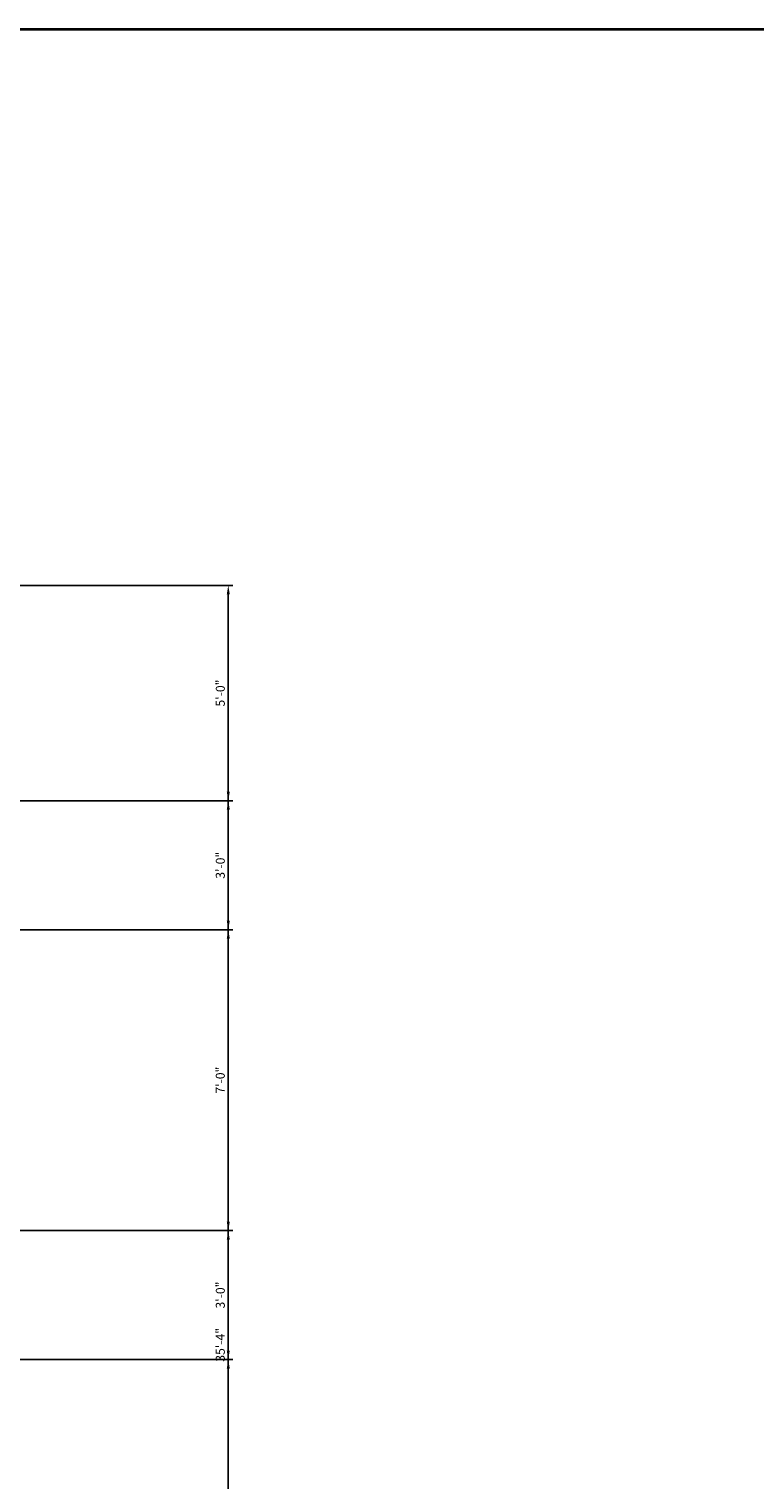
# Model space of a CAD drawing. Units: inches. Extents: x 2020 to 7901, y 1581 to 3943.
# Tile 8 of 17: x 2672 to 2875, y 2663 to 3067. Entities that reach past the tile are written whole.
import ezdxf

# ---------------------------------------------------------------- set-up
doc = ezdxf.new("R2010")
doc.units = ezdxf.units.IN
doc.layers.add('A-ANNO-DIMS', color=2, linetype='Continuous', lineweight=18)
doc.layers.add('A-ANNO-TTLB', color=7, linetype='Continuous', lineweight=35)
doc.styles.get("Standard").update_dxf_attribs({"font": 'arial.ttf'})
doc.dimstyles.new('ISO-25', dxfattribs={"dimtxt": 2.5, "dimasz": 2.5, "dimexe": 1.25, "dimexo": 0.625, "dimtad": 1, "dimdec": 1, "dimlunit": 3, "dimtxsty": 'Standard', "dimcen": 2.5, "dimadec": 0, "dimazin": 0, "dimtfac": 1, "dimtdec": 1, "dimtmove": 0, "dimatfit": 3, "dimfxl": 1, "dimarcsym": 0})

# ---------------------------------------------------------------- blocks, each defined once
blk = doc.blocks.new('*D63')
at = {"layer": 'A-ANNO-DIMS', "color": 0, "lineweight": -2, "transparency": 16777216}
for p, q in [((2666.99, 2911.95), (2728.83, 2911.95)), ((2727.58, 2490.45), (2727.58, 2909.45)), ((2666.99, 2487.95), (2728.83, 2487.95))]:
    blk.add_line(p, q, dxfattribs=at)
at = {"layer": 'A-ANNO-DIMS', "color": 0, "transparency": 16777216}
for points in [[(2727.17, 2909.45), (2728, 2909.45), (2727.58, 2911.95)], [(2727.17, 2490.45), (2728, 2490.45), (2727.58, 2487.95)]]:
    blk.add_solid(points, dxfattribs=at)
at = {"layer": 'DEFPOINTS', "color": 0, "transparency": 16777216}
for p in [(2666.36, 2911.95), (2727.58, 2911.95), (2666.36, 2487.95)]:
    blk.add_point(p, dxfattribs=at)
at = {"layer": 'A-ANNO-DIMS', "color": 0, "transparency": 16777216, "insert": (2725.68, 2699.95), "char_height": 2.5, "attachment_point": 5, "rotation": 90}
blk.add_mtext('35\'-4"', dxfattribs=at)
blk = doc.blocks.new('*D150')
at = {"layer": 'A-ANNO-DIMS', "color": 0, "lineweight": -2, "transparency": 16777216}
for p, q in [((2666.99, 2695.85), (2728.83, 2695.85)), ((2727.58, 2614.35), (2727.58, 2693.35)), ((2666.99, 2611.85), (2728.83, 2611.85))]:
    blk.add_line(p, q, dxfattribs=at)
at = {"layer": 'A-ANNO-DIMS', "color": 0, "transparency": 16777216}
for points in [[(2727.17, 2693.35), (2728, 2693.35), (2727.58, 2695.85)], [(2727.17, 2614.35), (2728, 2614.35), (2727.58, 2611.85)]]:
    blk.add_solid(points, dxfattribs=at)
at = {"layer": 'DEFPOINTS', "color": 0, "transparency": 16777216}
for p in [(2666.36, 2695.85), (2727.58, 2695.85), (2666.36, 2611.85)]:
    blk.add_point(p, dxfattribs=at)
at = {"layer": 'A-ANNO-DIMS', "color": 0, "transparency": 16777216, "insert": (2725.68, 2653.85), "char_height": 2.5, "attachment_point": 5, "rotation": 90}
blk.add_mtext('7\'-0"', dxfattribs=at)
blk = doc.blocks.new('*D151')
at = {"layer": 'A-ANNO-DIMS', "color": 0, "lineweight": -2, "transparency": 16777216}
for p, q in [((2666.99, 2731.85), (2728.83, 2731.85)), ((2727.58, 2698.35), (2727.58, 2729.35)), ((2666.99, 2695.85), (2728.83, 2695.85))]:
    blk.add_line(p, q, dxfattribs=at)
at = {"layer": 'A-ANNO-DIMS', "color": 0, "transparency": 16777216}
for points in [[(2727.17, 2729.35), (2728, 2729.35), (2727.58, 2731.85)], [(2727.17, 2698.35), (2728, 2698.35), (2727.58, 2695.85)]]:
    blk.add_solid(points, dxfattribs=at)
at = {"layer": 'DEFPOINTS', "color": 0, "transparency": 16777216}
for p in [(2666.36, 2731.85), (2727.58, 2731.85), (2666.36, 2695.85)]:
    blk.add_point(p, dxfattribs=at)
at = {"layer": 'A-ANNO-DIMS', "color": 0, "transparency": 16777216, "insert": (2725.68, 2713.85), "char_height": 2.5, "attachment_point": 5, "rotation": 90}
blk.add_mtext('3\'-0"', dxfattribs=at)
blk = doc.blocks.new('*D152')
at = {"layer": 'A-ANNO-DIMS', "color": 0, "lineweight": -2, "transparency": 16777216}
for p, q in [((2666.99, 2815.83), (2728.83, 2815.83)), ((2727.58, 2734.35), (2727.58, 2813.33)), ((2666.99, 2731.85), (2728.83, 2731.85))]:
    blk.add_line(p, q, dxfattribs=at)
at = {"layer": 'A-ANNO-DIMS', "color": 0, "transparency": 16777216}
for points in [[(2727.17, 2813.33), (2728, 2813.33), (2727.58, 2815.83)], [(2727.17, 2734.35), (2728, 2734.35), (2727.58, 2731.85)]]:
    blk.add_solid(points, dxfattribs=at)
at = {"layer": 'DEFPOINTS', "color": 0, "transparency": 16777216}
for p in [(2666.36, 2815.83), (2727.58, 2815.83), (2666.36, 2731.85)]:
    blk.add_point(p, dxfattribs=at)
at = {"layer": 'A-ANNO-DIMS', "color": 0, "transparency": 16777216, "insert": (2725.68, 2773.84), "char_height": 2.5, "attachment_point": 5, "rotation": 90}
blk.add_mtext('7\'-0"', dxfattribs=at)
blk = doc.blocks.new('*D153')
at = {"layer": 'A-ANNO-DIMS', "color": 0, "lineweight": -2, "transparency": 16777216}
for p, q in [((2666.99, 2851.83), (2728.83, 2851.83)), ((2727.58, 2818.33), (2727.58, 2849.33)), ((2666.99, 2815.83), (2728.83, 2815.83))]:
    blk.add_line(p, q, dxfattribs=at)
at = {"layer": 'A-ANNO-DIMS', "color": 0, "transparency": 16777216}
for points in [[(2727.17, 2849.33), (2728, 2849.33), (2727.58, 2851.83)], [(2727.17, 2818.33), (2728, 2818.33), (2727.58, 2815.83)]]:
    blk.add_solid(points, dxfattribs=at)
at = {"layer": 'DEFPOINTS', "color": 0, "transparency": 16777216}
for p in [(2666.36, 2851.83), (2727.58, 2851.83), (2666.36, 2815.83)]:
    blk.add_point(p, dxfattribs=at)
at = {"layer": 'A-ANNO-DIMS', "color": 0, "transparency": 16777216, "insert": (2725.68, 2833.83), "char_height": 2.5, "attachment_point": 5, "rotation": 90}
blk.add_mtext('3\'-0"', dxfattribs=at)
blk = doc.blocks.new('*D154')
at = {"layer": 'A-ANNO-DIMS', "color": 0, "lineweight": -2, "transparency": 16777216}
for p, q in [((2666.99, 2911.95), (2728.83, 2911.95)), ((2727.58, 2854.33), (2727.58, 2909.45)), ((2666.99, 2851.83), (2728.83, 2851.83))]:
    blk.add_line(p, q, dxfattribs=at)
at = {"layer": 'A-ANNO-DIMS', "color": 0, "transparency": 16777216}
for points in [[(2727.17, 2909.45), (2728, 2909.45), (2727.58, 2911.95)], [(2727.17, 2854.33), (2728, 2854.33), (2727.58, 2851.83)]]:
    blk.add_solid(points, dxfattribs=at)
at = {"layer": 'DEFPOINTS', "color": 0, "transparency": 16777216}
for p in [(2666.36, 2911.95), (2727.58, 2911.95), (2666.36, 2851.83)]:
    blk.add_point(p, dxfattribs=at)
at = {"layer": 'A-ANNO-DIMS', "color": 0, "transparency": 16777216, "insert": (2725.68, 2881.89), "char_height": 2.5, "attachment_point": 5, "rotation": 90}
blk.add_mtext('5\'-0"', dxfattribs=at)

msp = doc.modelspace()

# ---------------------------------------------------------------- linework, layer by layer
at = {"layer": 'A-ANNO-TTLB'}
msp.add_lwpolyline([(2019.8, 3067.25), (4199.03, 3067.25), (4199.03, 1580.73), (2019.8, 1580.73)], close=True, dxfattribs=at)

# ---------------------------------------------------------------- dimensions: what is measured, and where the dimension line sits
at = {"layer": 'A-ANNO-DIMS'}
for base, p1, p2, picture, middle in [((2727.58, 2911.95), (2666.36, 2487.95), (2666.36, 2911.95), '*D63', (2725.68, 2699.95)), ((2727.58, 2911.95), (2666.36, 2851.83), (2666.36, 2911.95), '*D154', (2725.68, 2881.89)), ((2727.58, 2851.83), (2666.36, 2815.83), (2666.36, 2851.83), '*D153', (2725.68, 2833.83)), ((2727.58, 2815.83), (2666.36, 2731.85), (2666.36, 2815.83), '*D152', (2725.68, 2773.84)), ((2727.58, 2731.85), (2666.36, 2695.85), (2666.36, 2731.85), '*D151', (2725.68, 2713.85)), ((2727.58, 2695.85), (2666.36, 2611.85), (2666.36, 2695.85), '*D150', (2725.68, 2653.85))]:
    dim = msp.add_linear_dim(base=base, p1=p1, p2=p2, angle=90, dimstyle='ISO-25', override={"dimdec": 1, "dimlfac": 1, "dimrnd": 0, "dimzin": 1, "dimdsep": 46, "dimlunit": 4, "dimfrac": 2}, dxfattribs=at)
    dim.commit()
    dim.dimension.update_dxf_attribs({"geometry": picture, "text_midpoint": middle})

doc.saveas('drawing.dxf')
